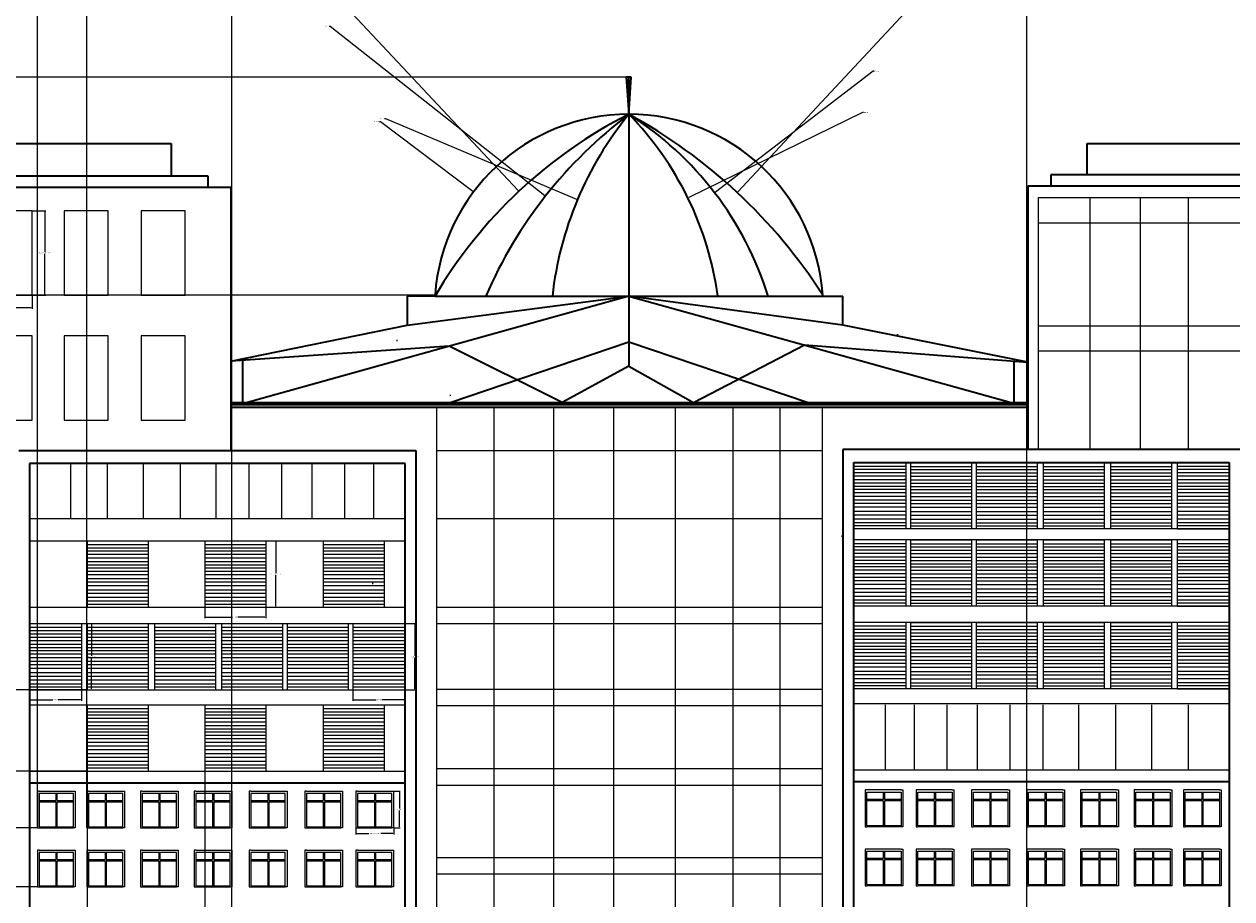
# Model space of a CAD drawing. Units: inches. Extents: x -279 to 364, y -385 to 335.
# Tile 7 of 9: x -60 to 168, y 34 to 199. Entities that reach past the tile are written whole.
import ezdxf

# ---------------------------------------------------------------- set-up
doc = ezdxf.new("R2010")
doc.units = ezdxf.units.IN
doc.header["$MEASUREMENT"] = 0
for name, color, linetype, lineweight in [('A-ANNO-DIMS', 2, 'Continuous', 18), ('A-GLAZ', 4, 'Continuous', 18), ('A-GLAZ-CURT', 4, 'Continuous', 18), ('A-ROOF', 7, 'Continuous', 35), ('A-WALL', 7, 'Continuous', 35), ('A-WALL-LOUV', 8, 'Continuous', 13)]:
    doc.layers.add(name, color=color, linetype=linetype, lineweight=lineweight)
doc.styles.get("Standard").update_dxf_attribs({"font": 'arial.ttf'})
doc.dimstyles.get("Standard").update_dxf_attribs({"dimtxt": 0.18, "dimasz": 0.18, "dimexe": 0.18, "dimexo": 0.0625, "dimgap": 0.09, "dimtad": 0, "dimtih": 1, "dimtoh": 1, "dimdec": 4, "dimzin": 0, "dimdsep": 46, "dimtxsty": 'Standard', "dimcen": 0.09, "dimadec": 0, "dimazin": 0, "dimtfac": 1, "dimtdec": 4, "dimtofl": 0, "dimtmove": 0, "dimatfit": 3, "dimfxl": 1, "dimtolj": 1, "dimtzin": 0, "dimarcsym": 0})

# ---------------------------------------------------------------- blocks, each defined once
blk = doc.blocks.new('WIN-TRANSOM-TWIN')
for p, q in [((0.32, 6.97), (0, 6.97)), ((0, 6.97), (0, 0)), ((0.32, 6.97), (6.81, 6.97)), ((6.81, 6.97), (7.13, 6.97)), ((7.13, 6.97), (7.13, 0)), ((0.32, 6.53), (0.32, 0.22)), ((6.81, 6.53), (0.32, 6.53)), ((0.32, 6.53), (0.32, 6.53)), ((0.32, 5.19), (3.48, 5.19)), ((0.32, 4.95), (3.48, 4.95)), ((3.48, 6.53), (3.48, 5.19)), ((3.48, 4.95), (3.48, 0.22)), ((3.69, 6.53), (3.69, 5.19)), ((3.69, 5.19), (6.81, 5.19)), ((3.69, 4.95), (3.69, 0.22)), ((3.69, 4.95), (6.81, 4.95)), ((6.81, 0.22), (6.81, 6.53)), ((0, 0), (0.32, 0)), ((0.32, 0.22), (6.81, 0.22)), ((0.32, 0), (6.81, 0)), ((7.13, 0), (6.81, 0))]:
    blk.add_line(p, q)
blk = doc.blocks.new('WIN-TOWER-FRONT')
for p, q in [((8.3, 15.93), (0, 15.93)), ((0, 15.93), (0, 14.74)), ((0, 14.74), (0, 0)), ((8.3, 0), (8.3, 15.93)), ((0, 0), (8.3, 0))]:
    blk.add_line(p, q)
blk = doc.blocks.new('LOUVER-FRONT-FIELD')
for p, q in [((0, 12.53), (11.53, 12.53)), ((0, 12.53), (0, 0)), ((0, 11.83), (11.53, 11.83)), ((11.53, 12.53), (11.53, 0)), ((0, 11.21), (11.53, 11.21)), ((0, 10.62), (11.53, 10.62)), ((0, 9.99), (11.53, 9.99)), ((0, 9.31), (11.53, 9.31)), ((0, 8.65), (11.53, 8.65)), ((0, 8), (11.53, 8)), ((0, 7.45), (11.53, 7.45)), ((0, 6.82), (11.53, 6.82)), ((0, 6.15), (11.53, 6.15)), ((0, 5.45), (11.53, 5.45)), ((0, 4.79), (11.53, 4.79)), ((0, 4.09), (11.53, 4.09)), ((0, 3.31), (11.53, 3.31)), ((0, 2.63), (11.53, 2.63)), ((0, 1.88), (11.53, 1.88)), ((0, 1.17), (11.53, 1.17)), ((0, 0.6), (11.53, 0.6))]:
    blk.add_line(p, q)
blk = doc.blocks.new('LOUVER-FRONT-END-A')
for p, q in [((0, 12.53), (9.8, 12.53)), ((0, 11.83), (9.8, 11.83)), ((9.8, 12.53), (9.8, 0)), ((0, 11.21), (9.8, 11.21)), ((0, 10.62), (9.8, 10.62)), ((0, 9.99), (9.8, 9.99)), ((0, 9.31), (9.8, 9.31)), ((0, 8.65), (9.8, 8.65)), ((0, 8), (9.8, 8)), ((0, 7.45), (9.8, 7.45)), ((0, 6.82), (9.8, 6.82)), ((0, 6.15), (9.8, 6.15)), ((0, 5.45), (9.8, 5.45)), ((0, 4.79), (9.8, 4.79)), ((0, 4.09), (9.8, 4.09)), ((0, 3.31), (9.8, 3.31)), ((0, 2.63), (9.8, 2.63)), ((0, 1.88), (9.8, 1.88)), ((0, 1.17), (9.8, 1.17)), ((0, 0.6), (9.8, 0.6)), ((9.8, 0), (0, 0))]:
    blk.add_line(p, q)
blk = doc.blocks.new('LOUVER-FRONT-END-B')
for p, q in [((0, 12.53), (9.83, 12.53)), ((0, 12.53), (0, 0)), ((0, 11.83), (9.83, 11.83)), ((0, 11.21), (9.83, 11.21)), ((0, 10.62), (9.83, 10.62)), ((0, 9.99), (9.83, 9.99)), ((0, 9.31), (9.83, 9.31)), ((0, 8.65), (9.83, 8.65)), ((0, 8), (9.83, 8)), ((0, 7.45), (9.83, 7.45)), ((0, 6.82), (9.83, 6.82)), ((0, 6.15), (9.83, 6.15)), ((0, 5.45), (9.83, 5.45)), ((0, 4.79), (9.83, 4.79)), ((0, 4.09), (9.83, 4.09)), ((0, 3.31), (9.83, 3.31)), ((0, 2.63), (9.83, 2.63)), ((0, 1.88), (9.83, 1.88)), ((0, 1.17), (9.83, 1.17)), ((0, 0.6), (9.83, 0.6))]:
    blk.add_line(p, q)
blk = doc.blocks.new('*D28')
at = {"layer": 'A-ANNO-DIMS', "color": 0, "lineweight": -2, "transparency": 16777216}
for p, q in [((2.24, 47.11), (2.24, 45.92)), ((2.42, 46.1), (4.68, 46.1)), ((9.19, 46.1), (6.93, 46.1)), ((9.37, 47.11), (9.37, 45.92))]:
    blk.add_line(p, q, dxfattribs=at)
at = {"layer": 'A-ANNO-DIMS', "color": 0, "transparency": 16777216}
for points in [[(2.42, 46.13), (2.42, 46.07), (2.24, 46.1)], [(9.19, 46.13), (9.19, 46.07), (9.37, 46.1)]]:
    blk.add_solid(points, dxfattribs=at)
at = {"layer": 'Defpoints', "color": 0, "transparency": 16777216}
for p in [(2.24, 47.17), (9.37, 47.17), (9.37, 46.1)]:
    blk.add_point(p, dxfattribs=at)
at = {"layer": 'A-ANNO-DIMS', "color": 0, "transparency": 16777216, "insert": (5.8, 46.1), "char_height": 0.18, "attachment_point": 5}
blk.add_mtext('\\A1;TRANSOM 7 TYP.', dxfattribs=at)
blk = doc.blocks.new('*D29')
at = {"layer": 'A-ANNO-DIMS', "color": 0, "lineweight": -2, "transparency": 16777216}
for p, q in [((9.43, 54.13), (10.62, 54.13)), ((10.44, 53.95), (10.44, 50.83)), ((10.44, 47.35), (10.44, 50.47)), ((9.43, 47.17), (10.62, 47.17))]:
    blk.add_line(p, q, dxfattribs=at)
at = {"layer": 'A-ANNO-DIMS', "color": 0, "transparency": 16777216}
for points in [[(10.41, 53.95), (10.47, 53.95), (10.44, 54.13)], [(10.41, 47.35), (10.47, 47.35), (10.44, 47.17)]]:
    blk.add_solid(points, dxfattribs=at)
at = {"layer": 'Defpoints', "color": 0, "transparency": 16777216}
for p in [(9.37, 54.13), (10.44, 54.13), (9.37, 47.17)]:
    blk.add_point(p, dxfattribs=at)
at = {"layer": 'A-ANNO-DIMS', "color": 0, "transparency": 16777216, "insert": (10.44, 50.65), "char_height": 0.18, "attachment_point": 5}
blk.add_mtext('\\A1;7 TYP.', dxfattribs=at)
blk = doc.blocks.new('*D34')
at = {"layer": 'A-ANNO-DIMS', "color": 0, "lineweight": -2, "transparency": 16777216}
for p, q in [((-58.87, 163.74), (-56.36, 163.74)), ((-56.54, 163.56), (-56.54, 155.96)), ((-56.54, 148), (-56.54, 155.6)), ((-58.87, 147.82), (-56.36, 147.82))]:
    blk.add_line(p, q, dxfattribs=at)
at = {"layer": 'A-ANNO-DIMS', "color": 0, "transparency": 16777216}
for points in [[(-56.57, 163.56), (-56.51, 163.56), (-56.54, 163.74)], [(-56.57, 148), (-56.51, 148), (-56.54, 147.82)]]:
    blk.add_solid(points, dxfattribs=at)
at = {"layer": 'Defpoints', "color": 0, "transparency": 16777216}
for p in [(-58.93, 163.74), (-56.54, 163.74), (-58.93, 147.82)]:
    blk.add_point(p, dxfattribs=at)
at = {"layer": 'A-ANNO-DIMS', "color": 0, "transparency": 16777216, "insert": (-56.54, 155.78), "char_height": 0.18, "attachment_point": 5}
blk.add_mtext('\\A1;TOWER SASH 16 TYP.', dxfattribs=at)
blk = doc.blocks.new('*D35')
at = {"layer": 'A-ANNO-DIMS', "color": 0, "lineweight": -2, "transparency": 16777216}
for p, q in [((-67.23, 147.75), (-67.23, 145.25)), ((-58.93, 147.75), (-58.93, 145.25)), ((-67.05, 145.43), (-63.54, 145.43)), ((-59.11, 145.43), (-62.62, 145.43))]:
    blk.add_line(p, q, dxfattribs=at)
at = {"layer": 'A-ANNO-DIMS', "color": 0, "transparency": 16777216}
for points in [[(-67.05, 145.46), (-67.05, 145.4), (-67.23, 145.43)], [(-59.11, 145.46), (-59.11, 145.4), (-58.93, 145.43)]]:
    blk.add_solid(points, dxfattribs=at)
at = {"layer": 'Defpoints', "color": 0, "transparency": 16777216}
for p in [(-67.23, 147.82), (-58.93, 147.82), (-58.93, 145.43)]:
    blk.add_point(p, dxfattribs=at)
at = {"layer": 'A-ANNO-DIMS', "color": 0, "transparency": 16777216, "insert": (-63.08, 145.43), "char_height": 0.18, "attachment_point": 5}
blk.add_mtext('\\A1;8 TYP.', dxfattribs=at)
blk = doc.blocks.new('*D40')
at = {"layer": 'A-ANNO-DIMS', "color": 0, "lineweight": -2, "transparency": 16777216}
for p, q in [((-14.74, 101.39), (-12.74, 101.39)), ((-12.92, 101.21), (-12.92, 95.31)), ((-12.92, 89.04), (-12.92, 94.94)), ((-14.74, 88.86), (-12.74, 88.86))]:
    blk.add_line(p, q, dxfattribs=at)
at = {"layer": 'A-ANNO-DIMS', "color": 0, "transparency": 16777216}
for points in [[(-12.95, 101.21), (-12.89, 101.21), (-12.92, 101.39)], [(-12.95, 89.04), (-12.89, 89.04), (-12.92, 88.86)]]:
    blk.add_solid(points, dxfattribs=at)
at = {"layer": 'Defpoints', "color": 0, "transparency": 16777216}
for p in [(-14.8, 101.39), (-12.92, 101.39), (-14.8, 88.86)]:
    blk.add_point(p, dxfattribs=at)
at = {"layer": 'A-ANNO-DIMS', "color": 0, "transparency": 16777216, "insert": (-12.92, 95.13), "char_height": 0.18, "attachment_point": 5}
blk.add_mtext('\\A1;FIELD LOUVER 13 TYP.', dxfattribs=at)
blk = doc.blocks.new('*D41')
at = {"layer": 'A-ANNO-DIMS', "color": 0, "lineweight": -2, "transparency": 16777216}
for p, q in [((-26.33, 88.8), (-26.33, 86.8)), ((-26.15, 86.98), (-21.09, 86.98)), ((-14.98, 86.98), (-20.05, 86.98)), ((-14.8, 88.8), (-14.8, 86.8))]:
    blk.add_line(p, q, dxfattribs=at)
at = {"layer": 'A-ANNO-DIMS', "color": 0, "transparency": 16777216}
for points in [[(-26.15, 87.01), (-26.15, 86.95), (-26.33, 86.98)], [(-14.98, 87.01), (-14.98, 86.95), (-14.8, 86.98)]]:
    blk.add_solid(points, dxfattribs=at)
at = {"layer": 'Defpoints', "color": 0, "transparency": 16777216}
for p in [(-26.33, 88.86), (-14.8, 88.86), (-14.8, 86.98)]:
    blk.add_point(p, dxfattribs=at)
at = {"layer": 'A-ANNO-DIMS', "color": 0, "transparency": 16777216, "insert": (-20.57, 86.98), "char_height": 0.18, "attachment_point": 5}
blk.add_mtext('\\A1;12 TYP.', dxfattribs=at)
blk = doc.blocks.new('*D42')
at = {"layer": 'A-ANNO-DIMS', "color": 0, "lineweight": -2, "transparency": 16777216}
for p, q in [((-49.56, 85.77), (-47.56, 85.77)), ((-47.74, 85.59), (-47.74, 79.68)), ((-47.74, 73.41), (-47.74, 79.32)), ((-49.56, 73.23), (-47.56, 73.23))]:
    blk.add_line(p, q, dxfattribs=at)
at = {"layer": 'A-ANNO-DIMS', "color": 0, "transparency": 16777216}
for points in [[(-47.77, 85.59), (-47.71, 85.59), (-47.74, 85.77)], [(-47.77, 73.41), (-47.71, 73.41), (-47.74, 73.23)]]:
    blk.add_solid(points, dxfattribs=at)
at = {"layer": 'Defpoints', "color": 0, "transparency": 16777216}
for p in [(-49.62, 85.77), (-47.74, 85.77), (-49.62, 73.23)]:
    blk.add_point(p, dxfattribs=at)
at = {"layer": 'A-ANNO-DIMS', "color": 0, "transparency": 16777216, "insert": (-47.74, 79.5), "char_height": 0.18, "attachment_point": 5}
blk.add_mtext('\\A1;END A 13 TYP.', dxfattribs=at)
blk = doc.blocks.new('*D43')
at = {"layer": 'A-ANNO-DIMS', "color": 0, "lineweight": -2, "transparency": 16777216}
for p, q in [((-59.43, 73.17), (-59.43, 71.17)), ((-49.62, 73.17), (-49.62, 71.17)), ((-59.25, 71.35), (-55.04, 71.35)), ((-49.8, 71.35), (-54.01, 71.35))]:
    blk.add_line(p, q, dxfattribs=at)
at = {"layer": 'A-ANNO-DIMS', "color": 0, "transparency": 16777216}
for points in [[(-59.25, 71.38), (-59.25, 71.32), (-59.43, 71.35)], [(-49.8, 71.38), (-49.8, 71.32), (-49.62, 71.35)]]:
    blk.add_solid(points, dxfattribs=at)
at = {"layer": 'Defpoints', "color": 0, "transparency": 16777216}
for p in [(-59.43, 73.23), (-49.62, 73.23), (-49.62, 71.35)]:
    blk.add_point(p, dxfattribs=at)
at = {"layer": 'A-ANNO-DIMS', "color": 0, "transparency": 16777216, "insert": (-54.53, 71.35), "char_height": 0.18, "attachment_point": 5}
blk.add_mtext('\\A1;10 TYP.', dxfattribs=at)
blk = doc.blocks.new('*D44')
at = {"layer": 'A-ANNO-DIMS', "color": 0, "lineweight": -2, "transparency": 16777216}
for p, q in [((11.57, 85.77), (13.57, 85.77)), ((13.39, 85.59), (13.39, 79.68)), ((13.39, 73.41), (13.39, 79.32)), ((11.57, 73.23), (13.57, 73.23))]:
    blk.add_line(p, q, dxfattribs=at)
at = {"layer": 'A-ANNO-DIMS', "color": 0, "transparency": 16777216}
for points in [[(13.36, 85.59), (13.42, 85.59), (13.39, 85.77)], [(13.36, 73.41), (13.42, 73.41), (13.39, 73.23)]]:
    blk.add_solid(points, dxfattribs=at)
at = {"layer": 'Defpoints', "color": 0, "transparency": 16777216}
for p in [(11.51, 85.77), (13.39, 85.77), (11.51, 73.23)]:
    blk.add_point(p, dxfattribs=at)
at = {"layer": 'A-ANNO-DIMS', "color": 0, "transparency": 16777216, "insert": (13.39, 79.5), "char_height": 0.18, "attachment_point": 5}
blk.add_mtext('\\A1;END B 13 TYP.', dxfattribs=at)
blk = doc.blocks.new('*D45')
at = {"layer": 'A-ANNO-DIMS', "color": 0, "lineweight": -2, "transparency": 16777216}
for p, q in [((1.68, 73.17), (1.68, 71.17)), ((11.51, 73.17), (11.51, 71.17)), ((1.86, 71.35), (6.08, 71.35)), ((11.33, 71.35), (7.12, 71.35))]:
    blk.add_line(p, q, dxfattribs=at)
at = {"layer": 'A-ANNO-DIMS', "color": 0, "transparency": 16777216}
for points in [[(1.86, 71.38), (1.86, 71.32), (1.68, 71.35)], [(11.33, 71.38), (11.33, 71.32), (11.51, 71.35)]]:
    blk.add_solid(points, dxfattribs=at)
at = {"layer": 'Defpoints', "color": 0, "transparency": 16777216}
for p in [(1.68, 73.23), (11.51, 73.23), (11.51, 71.35)]:
    blk.add_point(p, dxfattribs=at)
at = {"layer": 'A-ANNO-DIMS', "color": 0, "transparency": 16777216, "insert": (6.6, 71.35), "char_height": 0.18, "attachment_point": 5}
blk.add_mtext('\\A1;10 TYP.', dxfattribs=at)
blk = doc.blocks.new('*D74')
at = {"layer": 'A-ANNO-DIMS', "color": 0, "lineweight": -2, "transparency": 16777216}
for p, q in [((-137.56, 76.08), (-137.56, 213.67)), ((-137.38, 213.49), (54.29, 213.49)), ((246.75, 213.49), (55.08, 213.49)), ((246.93, 76.27), (246.93, 213.67))]:
    blk.add_line(p, q, dxfattribs=at)
at = {"layer": 'A-ANNO-DIMS', "color": 0, "transparency": 16777216}
for points in [[(-137.38, 213.52), (-137.38, 213.46), (-137.56, 213.49)], [(246.75, 213.52), (246.75, 213.46), (246.93, 213.49)]]:
    blk.add_solid(points, dxfattribs=at)
at = {"layer": 'Defpoints', "color": 0, "transparency": 16777216}
for p in [(246.93, 213.49), (-137.56, 76.01), (246.93, 76.21)]:
    blk.add_point(p, dxfattribs=at)
at = {"layer": 'A-ANNO-DIMS', "color": 0, "transparency": 16777216, "insert": (54.68, 213.49), "char_height": 0.18, "attachment_point": 5}
blk.add_mtext('\\A1;384.5', dxfattribs=at)
blk = doc.blocks.new('*D75')
at = {"layer": 'A-ANNO-DIMS', "color": 0, "lineweight": -2, "transparency": 16777216}
for p, q in [((53.76, 188.99), (-212.62, 188.99)), ((-212.44, 188.81), (-212.44, 84.64)), ((-212.44, -19.9), (-212.44, 84.27)), ((-133.86, -20.08), (-212.62, -20.08))]:
    blk.add_line(p, q, dxfattribs=at)
at = {"layer": 'A-ANNO-DIMS', "color": 0, "transparency": 16777216}
for points in [[(-212.47, 188.81), (-212.41, 188.81), (-212.44, 188.99)], [(-212.47, -19.9), (-212.41, -19.9), (-212.44, -20.08)]]:
    blk.add_solid(points, dxfattribs=at)
at = {"layer": 'Defpoints', "color": 0, "transparency": 16777216}
for p in [(-212.44, 188.99), (53.82, 188.99), (-133.8, -20.08)]:
    blk.add_point(p, dxfattribs=at)
at = {"layer": 'A-ANNO-DIMS', "color": 0, "transparency": 16777216, "insert": (-212.44, 84.45), "char_height": 0.18, "attachment_point": 5}
blk.add_mtext('\\A1;209.07', dxfattribs=at)
blk = doc.blocks.new('*D76')
at = {"layer": 'A-ANNO-DIMS', "color": 0, "lineweight": -2, "transparency": 16777216}
for p, q in [((17.12, 147.82), (-212.62, 147.82)), ((-212.44, 147.64), (-212.44, 64.05)), ((-212.44, -19.9), (-212.44, 63.68)), ((17.4, -20.08), (-212.62, -20.08))]:
    blk.add_line(p, q, dxfattribs=at)
at = {"layer": 'A-ANNO-DIMS', "color": 0, "transparency": 16777216}
for points in [[(-212.47, 147.64), (-212.41, 147.64), (-212.44, 147.82)], [(-212.47, -19.9), (-212.41, -19.9), (-212.44, -20.08)]]:
    blk.add_solid(points, dxfattribs=at)
at = {"layer": 'Defpoints', "color": 0, "transparency": 16777216}
for p in [(-212.44, 147.82), (17.19, 147.82), (17.46, -20.08)]:
    blk.add_point(p, dxfattribs=at)
at = {"layer": 'A-ANNO-DIMS', "color": 0, "transparency": 16777216, "insert": (-212.44, 63.87), "char_height": 0.18, "attachment_point": 5}
blk.add_mtext('\\A1;167.9', dxfattribs=at)
blk = doc.blocks.new('*D89')
at = {"layer": 'A-ANNO-DIMS', "color": 0, "lineweight": -2, "transparency": 16777216}
for p, q in [((-57.96, 47.23), (-57.96, 213.67)), ((-57.78, 213.49), (-53.69, 213.49)), ((-48.8, 213.49), (-52.9, 213.49)), ((-48.62, 47.23), (-48.62, 213.67))]:
    blk.add_line(p, q, dxfattribs=at)
at = {"layer": 'A-ANNO-DIMS', "color": 0, "transparency": 16777216}
for points in [[(-57.78, 213.52), (-57.78, 213.46), (-57.96, 213.49)], [(-48.8, 213.52), (-48.8, 213.46), (-48.62, 213.49)]]:
    blk.add_solid(points, dxfattribs=at)
at = {"layer": 'Defpoints', "color": 0, "transparency": 16777216}
for p in [(-48.62, 213.49), (-57.96, 47.17), (-48.62, 47.17)]:
    blk.add_point(p, dxfattribs=at)
at = {"layer": 'A-ANNO-DIMS', "color": 0, "transparency": 16777216, "insert": (-53.29, 213.49), "char_height": 0.18, "attachment_point": 5}
blk.add_mtext('\\A1;9.335', dxfattribs=at)
blk = doc.blocks.new('*D90')
at = {"layer": 'A-ANNO-DIMS', "color": 0, "lineweight": -2, "transparency": 16777216}
for p, q in [((-58.02, 47.17), (-212.62, 47.17)), ((-212.44, 46.99), (-212.44, 41.78)), ((-212.44, 36.2), (-212.44, 41.41)), ((-58.02, 36.02), (-212.62, 36.02))]:
    blk.add_line(p, q, dxfattribs=at)
at = {"layer": 'A-ANNO-DIMS', "color": 0, "transparency": 16777216}
for points in [[(-212.47, 46.99), (-212.41, 46.99), (-212.44, 47.17)], [(-212.47, 36.2), (-212.41, 36.2), (-212.44, 36.02)]]:
    blk.add_solid(points, dxfattribs=at)
at = {"layer": 'Defpoints', "color": 0, "transparency": 16777216}
for p in [(-57.96, 47.17), (-212.44, 36.02), (-57.96, 36.02)]:
    blk.add_point(p, dxfattribs=at)
at = {"layer": 'A-ANNO-DIMS', "color": 0, "transparency": 16777216, "insert": (-212.44, 41.59), "char_height": 0.18, "attachment_point": 5}
blk.add_mtext('\\A1;11.149', dxfattribs=at)
blk = doc.blocks.new('*D91')
at = {"layer": 'A-ANNO-DIMS', "color": 0, "lineweight": -2, "transparency": 16777216}
for p, q in [((-48.59, 73.23), (-212.62, 73.23)), ((-212.44, 73.05), (-212.44, 65.74)), ((-212.44, 58.07), (-212.44, 65.38)), ((-48.59, 57.89), (-212.62, 57.89))]:
    blk.add_line(p, q, dxfattribs=at)
at = {"layer": 'A-ANNO-DIMS', "color": 0, "transparency": 16777216}
for points in [[(-212.47, 73.05), (-212.41, 73.05), (-212.44, 73.23)], [(-212.47, 58.07), (-212.41, 58.07), (-212.44, 57.89)]]:
    blk.add_solid(points, dxfattribs=at)
at = {"layer": 'Defpoints', "color": 0, "transparency": 16777216}
for p in [(-212.44, 73.23), (-48.53, 73.23), (-48.53, 57.89)]:
    blk.add_point(p, dxfattribs=at)
at = {"layer": 'A-ANNO-DIMS', "color": 0, "transparency": 16777216, "insert": (-212.44, 65.56), "char_height": 0.18, "attachment_point": 5}
blk.add_mtext('\\A1;15.345', dxfattribs=at)
blk = doc.blocks.new('*D92')
at = {"layer": 'A-ANNO-DIMS', "color": 0, "lineweight": -2, "transparency": 16777216}
for p, q in [((-48.53, 57.83), (-48.53, -62.3)), ((-26.33, 57.83), (-26.33, -62.3)), ((-48.35, -62.12), (-37.75, -62.12)), ((-26.51, -62.12), (-37.11, -62.12))]:
    blk.add_line(p, q, dxfattribs=at)
at = {"layer": 'A-ANNO-DIMS', "color": 0, "transparency": 16777216}
for points in [[(-48.35, -62.09), (-48.35, -62.15), (-48.53, -62.12)], [(-26.51, -62.09), (-26.51, -62.15), (-26.33, -62.12)]]:
    blk.add_solid(points, dxfattribs=at)
at = {"layer": 'Defpoints', "color": 0, "transparency": 16777216}
for p in [(-48.53, 57.89), (-26.33, 57.89), (-26.33, -62.12)]:
    blk.add_point(p, dxfattribs=at)
at = {"layer": 'A-ANNO-DIMS', "color": 0, "transparency": 16777216, "insert": (-37.43, -62.12), "char_height": 0.18, "attachment_point": 5}
blk.add_mtext('\\A1;22.2', dxfattribs=at)
blk = doc.blocks.new('*D93')
at = {"layer": 'A-ANNO-DIMS', "color": 0, "lineweight": -2, "transparency": 16777216}
for p, q in [((-21.19, 7.14), (-21.19, 213.67)), ((-21.01, 213.49), (53.45, 213.49)), ((128.81, 213.49), (54.36, 213.49)), ((128.99, 7.33), (128.99, 213.67))]:
    blk.add_line(p, q, dxfattribs=at)
at = {"layer": 'A-ANNO-DIMS', "color": 0, "transparency": 16777216}
for points in [[(-21.01, 213.52), (-21.01, 213.46), (-21.19, 213.49)], [(128.81, 213.52), (128.81, 213.46), (128.99, 213.49)]]:
    blk.add_solid(points, dxfattribs=at)
at = {"layer": 'Defpoints', "color": 0, "transparency": 16777216}
for p in [(128.99, 213.49), (-21.19, 7.08), (128.99, 7.27)]:
    blk.add_point(p, dxfattribs=at)
at = {"layer": 'A-ANNO-DIMS', "color": 0, "transparency": 16777216, "insert": (53.9, 213.49), "char_height": 0.18, "attachment_point": 5}
blk.add_mtext('\\A1;150.18', dxfattribs=at)
blk = doc.blocks.new('*D117')
at = {"layer": 'A-ANNO-DIMS', "color": 0, "lineweight": -2, "transparency": 16777216}
for p, q in [((115.61, 211.52), (74.41, 167.34)), ((115.79, 211.52), (115.61, 211.52)), ((5.33, 93.35), (5.51, 93.35)), ((5.42, 93.26), (5.42, 93.44))]:
    blk.add_line(p, q, dxfattribs=at)
at = {"layer": 'A-ANNO-DIMS', "color": 0, "transparency": 16777216}
blk.add_solid([(74.39, 167.36), (74.44, 167.32), (74.29, 167.21)], dxfattribs=at)
at = {"layer": 'Defpoints', "color": 0, "transparency": 16777216}
for p in [(74.29, 167.21), (5.42, 93.35)]:
    blk.add_point(p, dxfattribs=at)
at = {"layer": 'A-ANNO-DIMS', "color": 0, "transparency": 16777216, "insert": (116.34, 211.52), "char_height": 0.18, "attachment_point": 5}
blk.add_mtext('\\A1;R100.98', dxfattribs=at)
blk = doc.blocks.new('*D118')
at = {"layer": 'A-ANNO-DIMS', "color": 0, "lineweight": -2, "transparency": 16777216}
for p, q in [((-3.78, 206.52), (-3.6, 206.52)), ((-3.6, 206.52), (32.92, 167.57)), ((94.02, 102.29), (94.2, 102.29)), ((94.11, 102.2), (94.11, 102.38))]:
    blk.add_line(p, q, dxfattribs=at)
at = {"layer": 'A-ANNO-DIMS', "color": 0, "transparency": 16777216}
blk.add_solid([(32.94, 167.59), (32.9, 167.55), (33.04, 167.44)], dxfattribs=at)
at = {"layer": 'Defpoints', "color": 0, "transparency": 16777216}
for p in [(33.04, 167.44), (94.11, 102.29)]:
    blk.add_point(p, dxfattribs=at)
at = {"layer": 'A-ANNO-DIMS', "color": 0, "transparency": 16777216, "insert": (-4.26, 206.52), "char_height": 0.18, "attachment_point": 5}
blk.add_mtext('\\A1;R89.29', dxfattribs=at)
blk = doc.blocks.new('*D119')
at = {"layer": 'A-ANNO-DIMS', "color": 0, "lineweight": -2, "transparency": 16777216}
for p, q in [((-2.83, 198.64), (-2.65, 198.64)), ((-2.65, 198.64), (37.94, 166.66)), ((105.88, 113.05), (106.06, 113.05)), ((105.97, 112.96), (105.97, 113.14))]:
    blk.add_line(p, q, dxfattribs=at)
at = {"layer": 'A-ANNO-DIMS', "color": 0, "transparency": 16777216}
blk.add_solid([(37.96, 166.68), (37.92, 166.63), (38.08, 166.55)], dxfattribs=at)
at = {"layer": 'Defpoints', "color": 0, "transparency": 16777216}
for p in [(38.08, 166.55), (105.97, 113.05)]:
    blk.add_point(p, dxfattribs=at)
at = {"layer": 'A-ANNO-DIMS', "color": 0, "transparency": 16777216, "insert": (-3.31, 198.64), "char_height": 0.18, "attachment_point": 5}
blk.add_mtext('\\A1;R86.43', dxfattribs=at)
blk = doc.blocks.new('*D120')
at = {"layer": 'A-ANNO-DIMS', "color": 0, "lineweight": -2, "transparency": 16777216}
for p, q in [((7.62, 181.15), (7.8, 181.15)), ((7.8, 181.15), (43.93, 165.93)), ((104.51, 140.37), (104.69, 140.37)), ((104.6, 140.28), (104.6, 140.46))]:
    blk.add_line(p, q, dxfattribs=at)
at = {"layer": 'A-ANNO-DIMS', "color": 0, "transparency": 16777216}
blk.add_solid([(43.95, 165.95), (43.92, 165.9), (44.1, 165.86)], dxfattribs=at)
at = {"layer": 'Defpoints', "color": 0, "transparency": 16777216}
for p in [(44.1, 165.86), (104.6, 140.37)]:
    blk.add_point(p, dxfattribs=at)
at = {"layer": 'A-ANNO-DIMS', "color": 0, "transparency": 16777216, "insert": (7.14, 181.15), "char_height": 0.18, "attachment_point": 5}
blk.add_mtext('\\A1;R65.65', dxfattribs=at)
blk = doc.blocks.new('*D121')
at = {"layer": 'A-ANNO-DIMS', "color": 0, "lineweight": -2, "transparency": 16777216}
for p, q in [((99.97, 190.09), (70.17, 167.25)), ((100.15, 190.09), (99.97, 190.09)), ((20.02, 128.9), (20.2, 128.9)), ((20.11, 128.81), (20.11, 128.99))]:
    blk.add_line(p, q, dxfattribs=at)
at = {"layer": 'A-ANNO-DIMS', "color": 0, "transparency": 16777216}
blk.add_solid([(70.15, 167.28), (70.19, 167.23), (70.03, 167.14)], dxfattribs=at)
at = {"layer": 'Defpoints', "color": 0, "transparency": 16777216}
for p in [(70.03, 167.14), (20.11, 128.9)]:
    blk.add_point(p, dxfattribs=at)
at = {"layer": 'A-ANNO-DIMS', "color": 0, "transparency": 16777216, "insert": (100.63, 190.09), "char_height": 0.18, "attachment_point": 5}
blk.add_mtext('\\A1;R62.88', dxfattribs=at)
blk = doc.blocks.new('*D122')
at = {"layer": 'A-ANNO-DIMS', "color": 0, "lineweight": -2, "transparency": 16777216}
for p, q in [((97.96, 182.3), (65.14, 166.23)), ((98.14, 182.3), (97.96, 182.3)), ((9.93, 139.25), (10.11, 139.25)), ((10.02, 139.16), (10.02, 139.34))]:
    blk.add_line(p, q, dxfattribs=at)
at = {"layer": 'A-ANNO-DIMS', "color": 0, "transparency": 16777216}
blk.add_solid([(65.13, 166.26), (65.15, 166.21), (64.98, 166.15)], dxfattribs=at)
at = {"layer": 'Defpoints', "color": 0, "transparency": 16777216}
for p in [(64.98, 166.15), (10.02, 139.25)]:
    blk.add_point(p, dxfattribs=at)
at = {"layer": 'A-ANNO-DIMS', "color": 0, "transparency": 16777216, "insert": (98.62, 182.3), "char_height": 0.18, "attachment_point": 5}
blk.add_mtext('\\A1;R61.19', dxfattribs=at)
blk = doc.blocks.new('*D123')
at = {"layer": 'A-ANNO-DIMS', "color": 0, "lineweight": -2, "transparency": 16777216}
for p, q in [((6.72, 180.62), (6.9, 180.62)), ((6.9, 180.62), (24.35, 167.47)), ((53.73, 145.25), (53.91, 145.25)), ((53.82, 145.16), (53.82, 145.34))]:
    blk.add_line(p, q, dxfattribs=at)
at = {"layer": 'A-ANNO-DIMS', "color": 0, "transparency": 16777216}
blk.add_solid([(24.37, 167.49), (24.33, 167.44), (24.49, 167.36)], dxfattribs=at)
at = {"layer": 'Defpoints', "color": 0, "transparency": 16777216}
for p in [(24.49, 167.36), (53.82, 145.25)]:
    blk.add_point(p, dxfattribs=at)
at = {"layer": 'A-ANNO-DIMS', "color": 0, "transparency": 16777216, "insert": (6.17, 180.62), "char_height": 0.18, "attachment_point": 5}
blk.add_mtext('\\A1;R36.724', dxfattribs=at)

msp = doc.modelspace()

# ---------------------------------------------------------------- linework, layer by layer
at = {"layer": 'A-GLAZ-CURT'}
for p, q in [((131.2105, 118.6379), (131.2105, 166.2338)), ((131.2105, 166.2338), (239.2791, 166.2338)), ((140.9288, 166.2338), (140.9288, 118.6379)), ((150.4123, 166.2338), (150.4123, 118.6379)), ((159.5311, 166.2338), (159.5311, 118.6379)), ((131.2105, 161.4639), (239.2791, 161.4639)), ((131.2105, 141.986), (239.2791, 141.986)), ((131.2105, 137.2845), (239.2791, 137.2845)), ((17.4585, 126.6636), (17.4585, 14.3396)), ((28.3065, 126.6636), (28.3065, 15.7643)), ((39.6009, 126.6636), (39.6009, 17.2476)), ((50.8952, 126.6636), (50.8952, 18.7309)), ((62.5929, 126.6636), (62.5929, 17.9201)), ((73.4839, 126.6636), (73.4839, 16.4361)), ((82.358, 126.6636), (82.358, 15.227)), ((90.3118, 126.6636), (90.3118, 68.1077)), ((17.4585, 118.4445), (90.3118, 118.4445)), ((-51.6968, 115.9949), (-51.6968, 105.61)), ((-44.759, 115.9949), (-44.759, 105.61)), ((-37.9547, 115.9949), (-37.9547, 105.61)), ((-30.964, 115.9949), (-30.964, 105.61)), ((-24.2529, 115.9949), (-24.2529, 105.61)), ((-18.0079, 115.9949), (-18.0079, 105.61)), ((-11.856, 115.9949), (-11.856, 105.61)), ((-6.0771, 115.9949), (-6.0771, 105.61)), ((0.0748, 115.9949), (0.0748, 105.61)), ((5.5741, 115.9949), (5.5741, 105.61)), ((-59.4257, 105.61), (11.51, 105.61)), ((17.4585, 105.61), (90.3118, 105.61)), ((17.4585, 88.8752), (90.3118, 88.8752)), ((17.4585, 85.7787), (90.3118, 85.7787)), ((17.4585, 73.3712), (90.3118, 73.3712)), ((17.4585, 70.2748), (90.3118, 70.2748)), ((167.2307, 70.6137), (96.295, 70.6137)), ((102.2308, 70.4361), (102.2308, 58.0818)), ((107.7302, 70.4361), (107.7302, 58.0818)), ((113.882, 70.4361), (113.882, 58.0818)), ((119.661, 70.4361), (119.661, 58.0818)), ((125.8128, 70.4361), (125.8128, 58.0818)), ((132.0579, 70.4361), (132.0579, 58.0818)), ((138.769, 70.4361), (138.769, 58.0818)), ((145.7597, 70.4361), (145.7597, 58.0818)), ((152.564, 70.4361), (152.564, 58.0818)), ((159.5017, 70.4361), (159.5017, 58.0818)), ((90.3118, 68.1077), (90.3118, 14.1432)), ((17.4585, 58.3621), (90.3118, 58.3621)), ((167.2307, 58.0818), (96.295, 58.0818)), ((17.4585, 55.2656), (90.3118, 55.2656)), ((17.4585, 41.5865), (90.3118, 41.5865)), ((17.4585, 38.49), (90.3118, 38.49))]:
    msp.add_line(p, q, dxfattribs=at)
at = {"layer": 'A-ROOF'}
for p, q in [((54.2707, 188.9896), (53.318, 188.9896)), ((53.318, 188.9896), (53.8218, 181.9792)), ((53.8218, 181.9792), (53.8218, 188.9896)), ((53.8218, 188.9896), (54.2707, 188.9896)), ((53.8218, 181.9792), (54.2707, 188.9896)), ((53.8218, 181.9792), (53.8218, 147.6369)), ((-90.5255, 176.4444), (-32.6709, 176.4444)), ((-32.6709, 176.4444), (-32.6709, 170.3156)), ((140.4124, 170.509), (140.4124, 176.4444)), ((140.4124, 176.4444), (198.2671, 176.4444)), ((-131.1712, 170.3156), (-25.7643, 170.3156)), ((-25.7643, 170.3156), (-25.7643, 168.1874)), ((238.9761, 170.509), (133.5692, 170.509)), ((133.5692, 170.509), (133.5692, 168.3808)), ((53.8218, 147.6369), (-18.2773, 127.5372)), ((17.1869, 147.6369), (11.9057, 147.6369)), ((11.9057, 147.6369), (11.9057, 142.132)), ((11.9057, 142.132), (53.8218, 147.6369)), ((17.1869, 147.6369), (90.4567, 147.6369)), ((53.8218, 147.6369), (126.0755, 127.5372)), ((94.2224, 142.132), (53.8218, 147.6369)), ((53.8218, 147.6369), (53.8218, 138.9612)), ((90.4567, 147.6369), (94.2224, 147.6369)), ((94.2224, 142.132), (94.2224, 147.6369)), ((-21.4109, 135.3084), (11.9057, 142.132)), ((129.2158, 135.1727), (94.2224, 142.132)), ((19.8617, 138.1695), (-21.4109, 135.3084)), ((41.2097, 127.5372), (19.8617, 138.1695)), ((20.0417, 127.5372), (53.8218, 138.9612)), ((53.8218, 138.9612), (87.7196, 127.5372)), ((53.8218, 138.9612), (53.8218, 134.3853)), ((66.0016, 127.5372), (87.0132, 138.4036)), ((87.0132, 138.4036), (129.2158, 135.1727)), ((-19.1978, 135.3084), (-19.1978, 127.5372)), ((126.5754, 135.3084), (126.5754, 127.5372)), ((53.8218, 134.3853), (41.2097, 127.5372)), ((53.8218, 134.3853), (66.0016, 127.5372)), ((-21.4109, 127.5372), (129.2158, 127.5372)), ((-21.4109, 127.1308), (129.2158, 127.1308)), ((-21.4109, 126.6636), (129.2158, 126.6636))]:
    msp.add_line(p, q, dxfattribs=at)
for centre, radius, start, end in [((53.8218, 145.2549), 36.7243, 3.997589, 176.002411), ((94.1065, 102.2938), 89.2895, 116.818707, 149.481201), ((105.9747, 113.0513), 86.4348, 127.112223, 156.413385), ((104.6035, 140.366), 65.6539, 140.667026, 173.641716), ((5.4193, 93.3518), 100.9832, 32.638073, 61.359517), ((10.0151, 139.2518), 61.1936, 7.875792, 44.285435), ((20.1113, 128.8952), 62.8833, 17.3399, 57.582834)]:
    msp.add_arc(centre, radius, start, end, dxfattribs=at)
at = {"layer": 'A-WALL'}
for p, q in [((-133.7987, 168.1874), (-21.4109, 168.1874)), ((-21.4109, 168.1874), (-21.4109, 118.4445)), ((129.2158, 168.3808), (129.2158, 118.6379)), ((241.6037, 168.3808), (129.2158, 168.3808)), ((-61.4888, 118.4445), (13.5848, 118.4445)), ((13.5848, 118.4445), (13.5848, 13.8309)), ((169.2937, 118.6379), (94.2202, 118.6379)), ((94.2202, 118.6379), (94.2202, 13.6107)), ((-58.3638, 115.9949), (-59.4257, 115.9949)), ((-59.4257, 115.9949), (-59.4257, -2.9883)), ((11.51, 115.9949), (-58.3638, 115.9949)), ((11.51, 13.5293), (11.51, 115.9949)), ((96.295, 116.1883), (166.1687, 116.1883)), ((96.295, 13.1982), (96.295, 116.1883)), ((166.1687, 116.1883), (167.2307, 116.1883)), ((167.2307, 116.1883), (167.2307, -2.7949)), ((-59.4257, 55.6745), (11.51, 55.6745)), ((167.2307, 55.8679), (96.295, 55.8679))]:
    msp.add_line(p, q, dxfattribs=at)
at = {"layer": 'A-WALL-LOUV'}
for p, q in [((157.4296, 116.1683), (96.295, 116.1683)), ((167.2307, 103.6363), (96.295, 103.6363)), ((-59.4257, 101.3936), (11.51, 101.3936)), ((157.4296, 101.5609), (96.295, 101.5609)), ((167.2307, 89.0551), (96.295, 89.0551)), ((167.2307, 89.0289), (96.295, 89.0289)), ((-59.4257, 88.8616), (11.51, 88.8616)), ((-49.6246, 85.7652), (11.51, 85.7652)), ((157.4296, 85.9586), (96.295, 85.9586)), ((-59.4257, 73.2332), (11.51, 73.2332)), ((167.2307, 73.4266), (96.295, 73.4266)), ((-59.4257, 70.4203), (11.51, 70.4203)), ((-59.4257, 57.8883), (11.51, 57.8883))]:
    msp.add_line(p, q, dxfattribs=at)

# ---------------------------------------------------------------- block references
at = {"layer": 'A-GLAZ'}
for name, p in [('WIN-TOWER-FRONT', (-67.2322, 147.815)), ('WIN-TOWER-FRONT', (-52.8939, 147.815)), ('WIN-TOWER-FRONT', (-38.3449, 147.815)), ('WIN-TOWER-FRONT', (-67.2322, 124.1691)), ('WIN-TOWER-FRONT', (-52.8939, 124.1691)), ('WIN-TOWER-FRONT', (-38.3449, 124.1691)), ('WIN-TRANSOM-TWIN', (-57.96, 47.168)), ('WIN-TRANSOM-TWIN', (-48.6248, 47.168)), ('WIN-TRANSOM-TWIN', (-38.5023, 47.168)), ('WIN-TRANSOM-TWIN', (-28.321, 47.168)), ('WIN-TRANSOM-TWIN', (-17.9147, 47.168)), ('WIN-TRANSOM-TWIN', (-7.4138, 47.168)), ('WIN-TRANSOM-TWIN', (2.2357, 47.168)), ('WIN-TRANSOM-TWIN', (-57.96, 36.0191)), ('WIN-TRANSOM-TWIN', (-48.6248, 36.0191)), ('WIN-TRANSOM-TWIN', (-38.5023, 36.0191)), ('WIN-TRANSOM-TWIN', (-28.321, 36.0191)), ('WIN-TRANSOM-TWIN', (-17.9147, 36.0191)), ('WIN-TRANSOM-TWIN', (-7.4138, 36.0191)), ('WIN-TRANSOM-TWIN', (2.2357, 36.0191))]:
    msp.add_blockref(name, p, dxfattribs=at)
at = {"layer": 'A-GLAZ', "extrusion": (0, 0, -1), "zscale": -1}
for p in [(-105.5693, 47.3614), (-115.2187, 47.3614), (-125.7196, 47.3614), (-136.1259, 47.3614), (-146.3073, 47.3614), (-156.4298, 47.3614), (-165.765, 47.3614), (-105.5693, 36.2126), (-115.2187, 36.2126), (-125.7196, 36.2126), (-136.1259, 36.2126), (-146.3073, 36.2126), (-156.4298, 36.2126), (-165.765, 36.2126)]:
    msp.add_blockref('WIN-TRANSOM-TWIN', p, dxfattribs=at)
at = {"layer": 'A-WALL-LOUV', "extrusion": (0, 0, -1), "zscale": -1}
for name, p in [('LOUVER-FRONT-END-B', (-106.124, 103.6361)), ('LOUVER-FRONT-END-A', (-167.231, 103.6361)), ('LOUVER-FRONT-END-B', (-106.124, 89.0287)), ('LOUVER-FRONT-END-A', (-167.231, 89.0287)), ('LOUVER-FRONT-END-B', (-106.124, 73.4264)), ('LOUVER-FRONT-END-A', (-167.231, 73.4264))]:
    msp.add_blockref(name, p, dxfattribs=at)
at = {"layer": 'A-WALL-LOUV'}
for name, p in [('LOUVER-FRONT-FIELD', (107.042, 103.636)), ('LOUVER-FRONT-FIELD', (119.4691, 103.636)), ('LOUVER-FRONT-FIELD', (132.0904, 103.636)), ('LOUVER-FRONT-FIELD', (144.8087, 103.636)), ('LOUVER-FRONT-FIELD', (-48.53, 88.8613)), ('LOUVER-FRONT-FIELD', (-26.3289, 88.8613)), ('LOUVER-FRONT-FIELD', (-3.9572, 88.8613)), ('LOUVER-FRONT-FIELD', (107.042, 89.0286)), ('LOUVER-FRONT-FIELD', (119.4691, 89.0286)), ('LOUVER-FRONT-FIELD', (132.0904, 89.0286)), ('LOUVER-FRONT-FIELD', (144.8087, 89.0286)), ('LOUVER-FRONT-END-A', (-59.426, 73.233)), ('LOUVER-FRONT-FIELD', (-48.53, 73.2329)), ('LOUVER-FRONT-FIELD', (-35.8116, 73.2329)), ('LOUVER-FRONT-FIELD', (-23.1904, 73.2329)), ('LOUVER-FRONT-FIELD', (-10.7633, 73.2329)), ('LOUVER-FRONT-END-B', (1.681, 73.233)), ('LOUVER-FRONT-FIELD', (107.042, 73.4263)), ('LOUVER-FRONT-FIELD', (119.4691, 73.4263)), ('LOUVER-FRONT-FIELD', (132.0904, 73.4263)), ('LOUVER-FRONT-FIELD', (144.8087, 73.4263)), ('LOUVER-FRONT-FIELD', (-48.53, 57.888)), ('LOUVER-FRONT-FIELD', (-26.3289, 57.888)), ('LOUVER-FRONT-FIELD', (-3.9572, 57.888))]:
    msp.add_blockref(name, p, dxfattribs=at)

# ---------------------------------------------------------------- dimensions: what is measured, and where the dimension line sits
at = {"layer": 'A-ANNO-DIMS'}
for base, p1, p2, override, picture, middle in [((246.9255, 213.4896), (-137.5587, 76.0128), (246.9255, 76.2063), {"dimdec": 1, "dimlfac": 1, "dimrnd": 0, "dimzin": 0, "dimdsep": 46, "dimlunit": 2}, '*D74', (54.6834, 213.4896)), ((-48.6244, 213.4896), (-57.9596, 47.1683), (-48.6244, 47.1683), {"dimdec": 3, "dimlfac": 1, "dimrnd": 0, "dimzin": 0, "dimdsep": 46, "dimlunit": 2}, '*D89', (-53.292, 213.4896)), ((128.9927, 213.4896), (-21.1877, 7.0763), (128.9927, 7.2697), {"dimdec": 2, "dimlfac": 1, "dimrnd": 0, "dimzin": 0, "dimdsep": 46, "dimlunit": 2}, '*D93', (53.9025, 213.4896)), ((-26.3293, -62.1247), (-48.5304, 57.8883), (-26.3293, 57.8883), {"dimdec": 1, "dimlfac": 1, "dimrnd": 0, "dimzin": 0, "dimdsep": 46, "dimlunit": 2}, '*D92', (-37.4299, -62.1247))]:
    dim = msp.add_linear_dim(base=base, p1=p1, p2=p2, dimstyle='Standard', override=override, dxfattribs=at)
    dim.commit()
    dim.dimension.update_dxf_attribs({"geometry": picture, "text_midpoint": middle})
for center, mpoint, override, picture, middle in [((5.4193, 93.3518), (74.291, 167.205), {"dimdec": 2, "dimlfac": 1, "dimrnd": 0, "dimzin": 0, "dimdsep": 46, "dimlunit": 2}, '*D117', (116.344, 211.517)), ((94.1065, 102.2938), (33.04, 167.436), {"dimdec": 2, "dimlfac": 1, "dimrnd": 0, "dimzin": 0, "dimdsep": 46, "dimlunit": 2}, '*D118', (-4.2599, 206.5213)), ((105.9747, 113.0513), (38.0838, 166.5471), {"dimdec": 2, "dimlfac": 1, "dimrnd": 0, "dimzin": 0, "dimdsep": 46, "dimlunit": 2}, '*D119', (-3.3105, 198.6447)), ((20.1113, 128.8952), (70.0261, 167.1421), {"dimdec": 2, "dimlfac": 1, "dimrnd": 0, "dimzin": 0, "dimdsep": 46, "dimlunit": 2}, '*D121', (100.635, 190.0902)), ((53.8218, 145.2549), (24.4935, 167.3574), {"dimdec": 3, "dimlfac": 1, "dimrnd": 0, "dimzin": 0, "dimdsep": 46, "dimlunit": 2}, '*D123', (6.1671, 180.6189)), ((104.6035, 140.366), (44.0998, 165.8561), {"dimdec": 2, "dimlfac": 1, "dimrnd": 0, "dimzin": 0, "dimdsep": 46, "dimlunit": 2}, '*D120', (7.1371, 181.1501)), ((10.0151, 139.2518), (64.9777, 166.1548), {"dimdec": 2, "dimlfac": 1, "dimrnd": 0, "dimzin": 0, "dimdsep": 46, "dimlunit": 2}, '*D122', (98.6152, 182.2967))]:
    dim = msp.add_radius_dim(center=center, mpoint=mpoint, dimstyle='Standard', override=override, dxfattribs=at)
    dim.commit()
    dim.dimension.update_dxf_attribs({"geometry": picture, "text_midpoint": middle, "dimtype": 164})
for base, p1, p2, override, picture, middle in [((-212.4386, 188.9896), (-133.7987, -20.0818), (53.8218, 188.9896), {"dimdec": 2, "dimlfac": 1, "dimrnd": 0, "dimzin": 0, "dimdsep": 46, "dimlunit": 2}, '*D75', (-212.4386, 84.4539)), ((-212.4386, 147.8151), (17.4585, -20.0818), (17.1869, 147.8151), {"dimdec": 1, "dimlfac": 1, "dimrnd": 0, "dimzin": 0, "dimdsep": 46, "dimlunit": 2}, '*D76', (-212.4386, 63.8666)), ((-212.4386, 73.2332), (-48.5304, 57.8883), (-48.5304, 73.2332), {"dimdec": 3, "dimlfac": 1, "dimrnd": 0, "dimzin": 0, "dimdsep": 46, "dimlunit": 2}, '*D91', (-212.4386, 65.5608)), ((-212.4386, 36.0194), (-57.9596, 47.1683), (-57.9596, 36.0194), {"dimdec": 3, "dimlfac": 1, "dimrnd": 0, "dimzin": 0, "dimdsep": 46, "dimlunit": 2}, '*D90', (-212.4386, 41.5939))]:
    dim = msp.add_linear_dim(base=base, p1=p1, p2=p2, angle=90, dimstyle='Standard', override=override, dxfattribs=at)
    dim.commit()
    dim.dimension.update_dxf_attribs({"geometry": picture, "text_midpoint": middle})
for base, p1, p2, text, picture, middle in [((-56.5401, 163.7435), (-58.9294, 147.8151), (-58.9294, 163.7435), 'TOWER SASH <> TYP.', '*D34', (-56.5401, 155.7793)), ((-12.9224, 101.3936), (-14.8022, 88.8616), (-14.8022, 101.3936), 'FIELD LOUVER <> TYP.', '*D40', (-12.9224, 95.1276)), ((-47.7448, 85.7652), (-49.6246, 73.2332), (-49.6246, 85.7652), 'END A <> TYP.', '*D42', (-47.7448, 79.4992)), ((13.3898, 85.7652), (11.51, 73.2332), (11.51, 85.7652), 'END B <> TYP.', '*D44', (13.3898, 79.4992)), ((10.4389, 54.1335), (9.369, 47.1683), (9.369, 54.1335), '<> TYP.', '*D29', (10.4389, 50.6509))]:
    dim = msp.add_linear_dim(base=base, p1=p1, p2=p2, angle=90, text=text, dimstyle='Standard', override={"dimdec": 0, "dimlfac": 1, "dimrnd": 0, "dimzin": 0, "dimdsep": 46, "dimlunit": 2}, dxfattribs=at)
    dim.commit()
    dim.dimension.update_dxf_attribs({"geometry": picture, "text_midpoint": middle})
for base, p1, p2, text, picture, middle in [((-58.9294, 145.4259), (-67.2327, 147.8151), (-58.9294, 147.8151), '<> TYP.', '*D35', (-63.081, 145.4259)), ((-14.8022, 86.9819), (-26.3293, 88.8616), (-14.8022, 88.8616), '<> TYP.', '*D41', (-20.5658, 86.9819)), ((-49.6246, 71.3534), (-59.4257, 73.2332), (-49.6246, 73.2332), '<> TYP.', '*D43', (-54.5252, 71.3534)), ((11.51, 71.3534), (1.6814, 73.2332), (11.51, 73.2332), '<> TYP.', '*D45', (6.5957, 71.3534)), ((9.369, 46.0984), (2.2361, 47.1683), (9.369, 47.1683), 'TRANSOM <> TYP.', '*D28', (5.8025, 46.0984))]:
    dim = msp.add_linear_dim(base=base, p1=p1, p2=p2, text=text, dimstyle='Standard', override={"dimdec": 0, "dimlfac": 1, "dimrnd": 0, "dimzin": 0, "dimdsep": 46, "dimlunit": 2}, dxfattribs=at)
    dim.commit()
    dim.dimension.update_dxf_attribs({"geometry": picture, "text_midpoint": middle})

doc.saveas('drawing.dxf')
